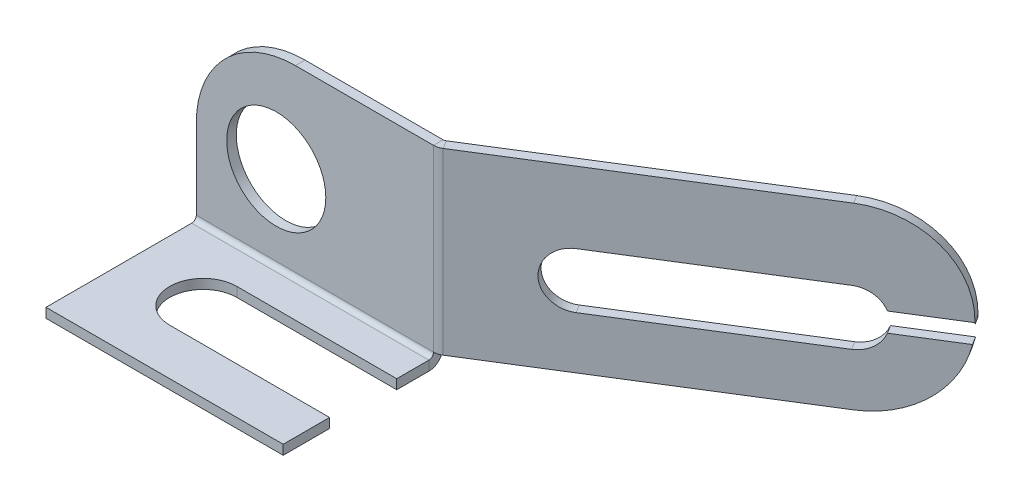
ISO-10303-21;
HEADER;
FILE_DESCRIPTION(('STEP AP214'),'2;1');
FILE_NAME('part.step','',(''),(''),'','','');
FILE_SCHEMA(('AUTOMOTIVE_DESIGN { 1 0 10303 214 1 1 1 1 }'));
ENDSEC;
DATA;
#1=APPLICATION_CONTEXT('core data for automotive mechanical design processes');
#2=APPLICATION_PROTOCOL_DEFINITION('international standard','automotive_design',2000,#1);
#3=PRODUCT_CONTEXT('',#1,'mechanical');
#4=PRODUCT('Part','Part','',(#3));
#5=PRODUCT_RELATED_PRODUCT_CATEGORY('part','',(#4));
#6=PRODUCT_DEFINITION_FORMATION('','',#4);
#7=PRODUCT_DEFINITION_CONTEXT('part definition',#1,'design');
#8=PRODUCT_DEFINITION('design','',#6,#7);
#9=PRODUCT_DEFINITION_SHAPE('','',#8);
#10=(LENGTH_UNIT() NAMED_UNIT(*) SI_UNIT(.MILLI.,.METRE.));
#11=(NAMED_UNIT(*) PLANE_ANGLE_UNIT() SI_UNIT($,.RADIAN.));
#12=(NAMED_UNIT(*) SI_UNIT($,.STERADIAN.) SOLID_ANGLE_UNIT());
#13=UNCERTAINTY_MEASURE_WITH_UNIT(LENGTH_MEASURE(1.E-05),#10,'distance_accuracy_value','');
#14=(GEOMETRIC_REPRESENTATION_CONTEXT(3) GLOBAL_UNCERTAINTY_ASSIGNED_CONTEXT((#13)) GLOBAL_UNIT_ASSIGNED_CONTEXT((#10,
#11,#12)) REPRESENTATION_CONTEXT('',''));
#15=CARTESIAN_POINT('',(0.,0.,0.));
#16=DIRECTION('',(0.,0.,1.));
#17=DIRECTION('',(1.,0.,0.));
#18=AXIS2_PLACEMENT_3D('',#15,#16,#17);
#19=CARTESIAN_POINT('',(37.6815119332738,23.1394,0.761999999999995));
#20=DIRECTION('',(1.,0.,0.));
#21=DIRECTION('',(0.,0.,-1.));
#22=AXIS2_PLACEMENT_3D('',#19,#20,#21);
#23=PLANE('',#22);
#24=DIRECTION('',(0.,1.,0.));
#25=VECTOR('',#24,1.);
#26=CARTESIAN_POINT('',(37.6815119332738,22.1234,6.604));
#27=LINE('',#26,#25);
#28=CARTESIAN_POINT('',(37.6815119332738,23.1394,6.604));
#29=VERTEX_POINT('',#28);
#30=CARTESIAN_POINT('',(37.6815119332738,24.6634,6.604));
#31=VERTEX_POINT('',#30);
#32=EDGE_CURVE('E267',#29,#31,#27,.T.);
#33=ORIENTED_EDGE('',*,*,#32,.F.);
#34=DIRECTION('',(0.,0.,-1.));
#35=VECTOR('',#34,1.);
#36=CARTESIAN_POINT('',(37.6815119332738,23.1394,0.761999999999995));
#37=LINE('',#36,#35);
#38=CARTESIAN_POINT('',(37.6815119332738,23.1394,1.49859999999999));
#39=VERTEX_POINT('',#38);
#40=EDGE_CURVE('E877',#29,#39,#37,.T.);
#41=ORIENTED_EDGE('',*,*,#40,.T.);
#42=DIRECTION('',(0.,-1.,0.));
#43=VECTOR('',#42,1.);
#44=CARTESIAN_POINT('',(37.6815119332738,24.6634,1.4986));
#45=LINE('',#44,#43);
#46=CARTESIAN_POINT('',(37.6815119332738,24.6634,1.4986));
#47=VERTEX_POINT('',#46);
#48=EDGE_CURVE('E283',#47,#39,#45,.T.);
#49=ORIENTED_EDGE('',*,*,#48,.F.);
#50=DIRECTION('',(0.,0.,1.));
#51=VECTOR('',#50,1.);
#52=CARTESIAN_POINT('',(37.6815119332738,24.6634,0.));
#53=LINE('',#52,#51);
#54=EDGE_CURVE('E271',#31,#47,#53,.F.);
#55=ORIENTED_EDGE('',*,*,#54,.F.);
#56=EDGE_LOOP('',(#33,#41,#49,#55));
#57=FACE_BOUND('',#56,.T.);
#58=ADVANCED_FACE('F69',(#57),#23,.T.);
#59=CARTESIAN_POINT('',(0.,12.7000000000001,-0.762));
#60=DIRECTION('',(-1.,0.,0.));
#61=DIRECTION('',(0.,0.,1.));
#62=AXIS2_PLACEMENT_3D('',#59,#60,#61);
#63=PLANE('',#62);
#64=DIRECTION('',(0.,-1.,0.));
#65=VECTOR('',#64,1.);
#66=CARTESIAN_POINT('',(0.,12.7000000000001,-0.762));
#67=LINE('',#66,#65);
#68=CARTESIAN_POINT('',(0.,38.0999999999999,-0.762));
#69=VERTEX_POINT('',#68);
#70=CARTESIAN_POINT('',(0.,25.4,-0.762));
#71=VERTEX_POINT('',#70);
#72=EDGE_CURVE('E351',#69,#71,#67,.T.);
#73=ORIENTED_EDGE('',*,*,#72,.T.);
#74=DIRECTION('',(0.,0.,1.));
#75=VECTOR('',#74,1.);
#76=CARTESIAN_POINT('',(0.,25.4,-0.762));
#77=LINE('',#76,#75);
#78=CARTESIAN_POINT('',(0.,25.4,0.761999999999998));
#79=VERTEX_POINT('',#78);
#80=EDGE_CURVE('E315',#79,#71,#77,.F.);
#81=ORIENTED_EDGE('',*,*,#80,.F.);
#82=DIRECTION('',(0.,-1.,0.));
#83=VECTOR('',#82,1.);
#84=CARTESIAN_POINT('',(0.,12.7000000000001,0.762));
#85=LINE('',#84,#83);
#86=CARTESIAN_POINT('',(0.,38.0999999999999,0.762));
#87=VERTEX_POINT('',#86);
#88=EDGE_CURVE('E336',#87,#79,#85,.T.);
#89=ORIENTED_EDGE('',*,*,#88,.F.);
#90=DIRECTION('',(0.,0.,1.));
#91=VECTOR('',#90,1.);
#92=CARTESIAN_POINT('',(0.,38.0999999999999,-0.762));
#93=LINE('',#92,#91);
#94=EDGE_CURVE('E356',#69,#87,#93,.T.);
#95=ORIENTED_EDGE('',*,*,#94,.F.);
#96=EDGE_LOOP('',(#73,#81,#89,#95));
#97=FACE_BOUND('',#96,.T.);
#98=ADVANCED_FACE('F511',(#97),#63,.T.);
#99=CARTESIAN_POINT('',(15.748,38.1,-0.762));
#100=DIRECTION('',(0.,0.,1.));
#101=DIRECTION('',(1.,0.,0.));
#102=AXIS2_PLACEMENT_3D('',#99,#100,#101);
#103=PLANE('',#102);
#104=CARTESIAN_POINT('',(12.7,38.1,-0.762));
#105=DIRECTION('',(0.,0.,1.));
#106=DIRECTION('',(1.,0.,0.));
#107=AXIS2_PLACEMENT_3D('',#104,#105,#106);
#108=CIRCLE('',#107,7.874);
#109=CARTESIAN_POINT('',(20.574,38.1,-0.762));
#110=VERTEX_POINT('',#109);
#111=EDGE_CURVE('E346',#110,#110,#108,.T.);
#112=ORIENTED_EDGE('',*,*,#111,.T.);
#113=EDGE_LOOP('',(#112));
#114=FACE_BOUND('',#113,.T.);
#115=DIRECTION('',(-1.,0.,0.));
#116=VECTOR('',#115,1.);
#117=CARTESIAN_POINT('',(15.748,25.4,-0.762));
#118=LINE('',#117,#116);
#119=CARTESIAN_POINT('',(37.6815119332738,25.4,-0.762000000000002));
#120=VERTEX_POINT('',#119);
#121=EDGE_CURVE('E307',#120,#71,#118,.T.);
#122=ORIENTED_EDGE('',*,*,#121,.T.);
#123=ORIENTED_EDGE('',*,*,#72,.F.);
#124=CARTESIAN_POINT('',(15.748,38.1,-0.762));
#125=DIRECTION('',(0.,0.,1.));
#126=DIRECTION('',(1.,0.,0.));
#127=AXIS2_PLACEMENT_3D('',#124,#125,#126);
#128=CIRCLE('',#127,15.748);
#129=CARTESIAN_POINT('',(15.7480000000001,53.848,-0.762));
#130=VERTEX_POINT('',#129);
#131=EDGE_CURVE('E359',#130,#69,#128,.T.);
#132=ORIENTED_EDGE('',*,*,#131,.F.);
#133=DIRECTION('',(-1.,0.,0.));
#134=VECTOR('',#133,1.);
#135=CARTESIAN_POINT('',(15.7480000000001,53.848,-0.762));
#136=LINE('',#135,#134);
#137=CARTESIAN_POINT('',(37.6815119332738,53.848,-0.762));
#138=VERTEX_POINT('',#137);
#139=EDGE_CURVE('E337',#138,#130,#136,.T.);
#140=ORIENTED_EDGE('',*,*,#139,.F.);
#141=DIRECTION('',(0.,-1.,0.));
#142=VECTOR('',#141,1.);
#143=CARTESIAN_POINT('',(37.6815119332738,38.1,-0.762));
#144=LINE('',#143,#142);
#145=EDGE_CURVE('E347',#138,#120,#144,.T.);
#146=ORIENTED_EDGE('',*,*,#145,.T.);
#147=EDGE_LOOP('',(#122,#123,#132,#140,#146));
#148=FACE_BOUND('',#147,.T.);
#149=ADVANCED_FACE('F519',(#114,#148),#103,.F.);
#150=CARTESIAN_POINT('',(15.748,38.1,0.762));
#151=DIRECTION('',(0.,0.,1.));
#152=DIRECTION('',(1.,0.,0.));
#153=AXIS2_PLACEMENT_3D('',#150,#151,#152);
#154=PLANE('',#153);
#155=CARTESIAN_POINT('',(12.7,38.1,0.762));
#156=DIRECTION('',(0.,0.,1.));
#157=DIRECTION('',(1.,0.,0.));
#158=AXIS2_PLACEMENT_3D('',#155,#156,#157);
#159=CIRCLE('',#158,7.874);
#160=CARTESIAN_POINT('',(20.574,38.1,0.762));
#161=VERTEX_POINT('',#160);
#162=EDGE_CURVE('E354',#161,#161,#159,.T.);
#163=ORIENTED_EDGE('',*,*,#162,.F.);
#164=EDGE_LOOP('',(#163));
#165=FACE_BOUND('',#164,.T.);
#166=ORIENTED_EDGE('',*,*,#88,.T.);
#167=DIRECTION('',(1.,0.,0.));
#168=VECTOR('',#167,1.);
#169=CARTESIAN_POINT('',(19.05,25.4,0.762));
#170=LINE('',#169,#168);
#171=CARTESIAN_POINT('',(37.6815119332738,25.4,0.761999999999998));
#172=VERTEX_POINT('',#171);
#173=EDGE_CURVE('E296',#172,#79,#170,.F.);
#174=ORIENTED_EDGE('',*,*,#173,.F.);
#175=DIRECTION('',(0.,-1.,0.));
#176=VECTOR('',#175,1.);
#177=CARTESIAN_POINT('',(37.6815119332738,38.1,0.762));
#178=LINE('',#177,#176);
#179=CARTESIAN_POINT('',(37.6815119332738,53.848,0.762));
#180=VERTEX_POINT('',#179);
#181=EDGE_CURVE('E361',#180,#172,#178,.T.);
#182=ORIENTED_EDGE('',*,*,#181,.F.);
#183=DIRECTION('',(-1.,0.,0.));
#184=VECTOR('',#183,1.);
#185=CARTESIAN_POINT('',(15.7480000000001,53.848,0.762));
#186=LINE('',#185,#184);
#187=CARTESIAN_POINT('',(15.7480000000001,53.848,0.762));
#188=VERTEX_POINT('',#187);
#189=EDGE_CURVE('E343',#180,#188,#186,.T.);
#190=ORIENTED_EDGE('',*,*,#189,.T.);
#191=CARTESIAN_POINT('',(15.748,38.1,0.762));
#192=DIRECTION('',(0.,0.,1.));
#193=DIRECTION('',(1.,0.,0.));
#194=AXIS2_PLACEMENT_3D('',#191,#192,#193);
#195=CIRCLE('',#194,15.748);
#196=EDGE_CURVE('E341',#188,#87,#195,.T.);
#197=ORIENTED_EDGE('',*,*,#196,.T.);
#198=EDGE_LOOP('',(#166,#174,#182,#190,#197));
#199=FACE_BOUND('',#198,.T.);
#200=ADVANCED_FACE('F500',(#165,#199),#154,.T.);
#201=CARTESIAN_POINT('',(37.6815119332738,71.797180792828,-1.4986));
#202=DIRECTION('',(0.,-1.,0.));
#203=DIRECTION('',(0.,0.,-1.));
#204=AXIS2_PLACEMENT_3D('',#201,#202,#203);
#205=CYLINDRICAL_SURFACE('',#204,0.7366);
#206=CARTESIAN_POINT('',(37.6815119332738,25.4,-1.4986));
#207=DIRECTION('',(0.,-1.,0.));
#208=DIRECTION('',(0.,0.,1.));
#209=AXIS2_PLACEMENT_3D('',#206,#207,#208);
#210=CIRCLE('',#209,0.7366);
#211=CARTESIAN_POINT('',(38.071850463308,25.4,-0.873927772371178));
#212=VERTEX_POINT('',#211);
#213=EDGE_CURVE('E322',#212,#120,#210,.T.);
#214=ORIENTED_EDGE('',*,*,#213,.T.);
#215=ORIENTED_EDGE('',*,*,#145,.F.);
#216=CARTESIAN_POINT('',(37.6815119332738,53.848,-1.4986));
#217=DIRECTION('',(0.,1.,0.));
#218=DIRECTION('',(0.,0.,-1.));
#219=AXIS2_PLACEMENT_3D('',#216,#217,#218);
#220=CIRCLE('',#219,0.7366);
#221=CARTESIAN_POINT('',(38.071850463308,53.848,-0.873927772371177));
#222=VERTEX_POINT('',#221);
#223=EDGE_CURVE('E318',#138,#222,#220,.T.);
#224=ORIENTED_EDGE('',*,*,#223,.T.);
#225=DIRECTION('',(0.,-1.,0.));
#226=VECTOR('',#225,1.);
#227=CARTESIAN_POINT('',(38.071850463308,38.1,-0.873927772371177));
#228=LINE('',#227,#226);
#229=EDGE_CURVE('E459',#222,#212,#228,.T.);
#230=ORIENTED_EDGE('',*,*,#229,.T.);
#231=EDGE_LOOP('',(#214,#215,#224,#230));
#232=FACE_BOUND('',#231,.T.);
#233=ADVANCED_FACE('F529',(#232),#205,.F.);
#234=CARTESIAN_POINT('',(37.6815119332738,71.797180792828,-1.4986));
#235=DIRECTION('',(0.,-1.,0.));
#236=DIRECTION('',(0.,0.,-1.));
#237=AXIS2_PLACEMENT_3D('',#234,#235,#236);
#238=CYLINDRICAL_SURFACE('',#237,2.2606);
#239=ORIENTED_EDGE('',*,*,#181,.T.);
#240=CARTESIAN_POINT('',(37.6815119332738,25.4,-1.4986));
#241=DIRECTION('',(0.,-1.,0.));
#242=DIRECTION('',(0.,0.,-1.));
#243=AXIS2_PLACEMENT_3D('',#240,#241,#242);
#244=CIRCLE('',#243,2.2606);
#245=CARTESIAN_POINT('',(38.8794474219994,25.4,0.418497526171215));
#246=VERTEX_POINT('',#245);
#247=EDGE_CURVE('E323',#246,#172,#244,.T.);
#248=ORIENTED_EDGE('',*,*,#247,.F.);
#249=DIRECTION('',(0.,-1.,0.));
#250=VECTOR('',#249,1.);
#251=CARTESIAN_POINT('',(38.8794474219994,38.1,0.418497526171215));
#252=LINE('',#251,#250);
#253=CARTESIAN_POINT('',(38.8794474219994,53.848,0.418497526171215));
#254=VERTEX_POINT('',#253);
#255=EDGE_CURVE('E77',#254,#246,#252,.T.);
#256=ORIENTED_EDGE('',*,*,#255,.F.);
#257=CARTESIAN_POINT('',(37.6815119332738,53.848,-1.4986));
#258=DIRECTION('',(0.,-1.,0.));
#259=DIRECTION('',(0.,0.,-1.));
#260=AXIS2_PLACEMENT_3D('',#257,#258,#259);
#261=CIRCLE('',#260,2.2606);
#262=EDGE_CURVE('E316',#180,#254,#261,.F.);
#263=ORIENTED_EDGE('',*,*,#262,.F.);
#264=EDGE_LOOP('',(#239,#248,#256,#263));
#265=FACE_BOUND('',#264,.T.);
#266=ADVANCED_FACE('F494',(#265),#238,.T.);
#267=CARTESIAN_POINT('',(78.2129451427182,25.4,-25.9568675896253));
#268=DIRECTION('',(0.,-1.,0.));
#269=DIRECTION('',(-0.529919264233206,0.,-0.848048096156425));
#270=AXIS2_PLACEMENT_3D('',#267,#268,#269);
#271=PLANE('',#270);
#272=DIRECTION('',(0.848048096156425,0.,-0.529919264233206));
#273=VECTOR('',#272,1.);
#274=CARTESIAN_POINT('',(79.0205421014096,25.4,-24.6644422910829));
#275=LINE('',#274,#273);
#276=CARTESIAN_POINT('',(79.0205421014096,25.4,-24.6644422910829));
#277=VERTEX_POINT('',#276);
#278=EDGE_CURVE('E428',#246,#277,#275,.T.);
#279=ORIENTED_EDGE('',*,*,#278,.F.);
#280=DIRECTION('',(-0.529919264233206,0.,-0.848048096156425));
#281=VECTOR('',#280,1.);
#282=CARTESIAN_POINT('',(38.071850463308,25.4,-0.873927772371177));
#283=LINE('',#282,#281);
#284=EDGE_CURVE('E458',#246,#212,#283,.T.);
#285=ORIENTED_EDGE('',*,*,#284,.T.);
#286=DIRECTION('',(0.848048096156425,0.,-0.529919264233206));
#287=VECTOR('',#286,1.);
#288=CARTESIAN_POINT('',(78.2129451427182,25.4,-25.9568675896253));
#289=LINE('',#288,#287);
#290=CARTESIAN_POINT('',(78.2129451427182,25.4,-25.9568675896253));
#291=VERTEX_POINT('',#290);
#292=EDGE_CURVE('E72',#212,#291,#289,.T.);
#293=ORIENTED_EDGE('',*,*,#292,.T.);
#294=DIRECTION('',(0.529919264233206,0.,0.848048096156425));
#295=VECTOR('',#294,1.);
#296=CARTESIAN_POINT('',(78.2129451427182,25.4,-25.9568675896253));
#297=LINE('',#296,#295);
#298=EDGE_CURVE('E455',#291,#277,#297,.T.);
#299=ORIENTED_EDGE('',*,*,#298,.T.);
#300=EDGE_LOOP('',(#279,#285,#293,#299));
#301=FACE_BOUND('',#300,.T.);
#302=ADVANCED_FACE('F466',(#301),#271,.T.);
#303=CARTESIAN_POINT('',(19.5689783684596,38.1,12.4850178087218));
#304=DIRECTION('',(0.529919264233206,0.,0.848048096156425));
#305=DIRECTION('',(0.848048096156425,0.,-0.529919264233206));
#306=AXIS2_PLACEMENT_3D('',#303,#304,#305);
#307=PLANE('',#306);
#308=DIRECTION('',(-0.848048096156425,0.,0.529919264233206));
#309=VECTOR('',#308,1.);
#310=CARTESIAN_POINT('',(19.5689783684597,53.848,12.4850178087217));
#311=LINE('',#310,#309);
#312=CARTESIAN_POINT('',(79.0205421014096,53.848,-24.6644422910829));
#313=VERTEX_POINT('',#312);
#314=EDGE_CURVE('E94',#313,#254,#311,.T.);
#315=ORIENTED_EDGE('',*,*,#314,.T.);
#316=ORIENTED_EDGE('',*,*,#255,.T.);
#317=ORIENTED_EDGE('',*,*,#278,.T.);
#318=CARTESIAN_POINT('',(79.0205421014097,39.37,-24.6644422910829));
#319=DIRECTION('',(0.529919264233206,0.,0.848048096156425));
#320=DIRECTION('',(0.848048096156425,0.,-0.529919264233206));
#321=AXIS2_PLACEMENT_3D('',#318,#319,#320);
#322=CIRCLE('',#321,13.97);
#323=CARTESIAN_POINT('',(90.6284113124176,36.576,-31.9178440020137));
#324=VERTEX_POINT('',#323);
#325=EDGE_CURVE('E440',#277,#324,#322,.T.);
#326=ORIENTED_EDGE('',*,*,#325,.T.);
#327=DIRECTION('',(0.848048096156425,0.,-0.529919264233206));
#328=VECTOR('',#327,1.);
#329=CARTESIAN_POINT('',(82.3080740718898,36.576,-26.718720262858));
#330=LINE('',#329,#328);
#331=CARTESIAN_POINT('',(82.3080740718898,36.576,-26.718720262858));
#332=VERTEX_POINT('',#331);
#333=EDGE_CURVE('E374',#332,#324,#330,.T.);
#334=ORIENTED_EDGE('',*,*,#333,.F.);
#335=CARTESIAN_POINT('',(78.805137884986,38.1,-24.5298427979677));
#336=DIRECTION('',(0.529919264233206,0.,0.848048096156425));
#337=DIRECTION('',(0.848048096156425,0.,-0.529919264233206));
#338=AXIS2_PLACEMENT_3D('',#335,#336,#337);
#339=CIRCLE('',#338,4.40276305129233);
#340=CARTESIAN_POINT('',(78.805137884986,33.6972369487077,-24.5298427979677));
#341=VERTEX_POINT('',#340);
#342=EDGE_CURVE('E375',#341,#332,#339,.T.);
#343=ORIENTED_EDGE('',*,*,#342,.F.);
#344=DIRECTION('',(0.848048096156425,0.,-0.529919264233206));
#345=VECTOR('',#344,1.);
#346=CARTESIAN_POINT('',(51.8796108320195,33.6972369487077,-7.70490615856339));
#347=LINE('',#346,#345);
#348=CARTESIAN_POINT('',(51.8796108320195,33.6972369487077,-7.7049061585634));
#349=VERTEX_POINT('',#348);
#350=EDGE_CURVE('E367',#349,#341,#347,.T.);
#351=ORIENTED_EDGE('',*,*,#350,.F.);
#352=CARTESIAN_POINT('',(51.8796108320195,38.1,-7.70490615856339));
#353=DIRECTION('',(0.529919264233206,0.,0.848048096156425));
#354=DIRECTION('',(0.848048096156425,0.,-0.529919264233206));
#355=AXIS2_PLACEMENT_3D('',#352,#353,#354);
#356=CIRCLE('',#355,4.40276305129234);
#357=CARTESIAN_POINT('',(51.8796108320195,42.5027630512923,-7.70490615856339));
#358=VERTEX_POINT('',#357);
#359=EDGE_CURVE('E331',#358,#349,#356,.T.);
#360=ORIENTED_EDGE('',*,*,#359,.F.);
#361=DIRECTION('',(0.848048096156425,0.,-0.529919264233206));
#362=VECTOR('',#361,1.);
#363=CARTESIAN_POINT('',(51.8796108320195,42.5027630512923,-7.70490615856339));
#364=LINE('',#363,#362);
#365=CARTESIAN_POINT('',(78.805137884986,42.5027630512923,-24.5298427979677));
#366=VERTEX_POINT('',#365);
#367=EDGE_CURVE('E384',#358,#366,#364,.T.);
#368=ORIENTED_EDGE('',*,*,#367,.T.);
#369=CARTESIAN_POINT('',(78.805137884986,38.1,-24.5298427979677));
#370=DIRECTION('',(0.529919264233206,0.,0.848048096156425));
#371=DIRECTION('',(0.848048096156425,0.,-0.529919264233206));
#372=AXIS2_PLACEMENT_3D('',#369,#370,#371);
#373=CIRCLE('',#372,4.40276305129233);
#374=CARTESIAN_POINT('',(82.3080740718898,39.624,-26.718720262858));
#375=VERTEX_POINT('',#374);
#376=EDGE_CURVE('E379',#375,#366,#373,.T.);
#377=ORIENTED_EDGE('',*,*,#376,.F.);
#378=DIRECTION('',(0.848048096156425,0.,-0.529919264233206));
#379=VECTOR('',#378,1.);
#380=CARTESIAN_POINT('',(82.3080740718898,39.624,-26.718720262858));
#381=LINE('',#380,#379);
#382=CARTESIAN_POINT('',(90.8658156227025,39.624,-32.0661906795219));
#383=VERTEX_POINT('',#382);
#384=EDGE_CURVE('E380',#375,#383,#381,.T.);
#385=ORIENTED_EDGE('',*,*,#384,.T.);
#386=CARTESIAN_POINT('',(79.0205421014097,39.37,-24.6644422910829));
#387=DIRECTION('',(0.529919264233206,0.,0.848048096156425));
#388=DIRECTION('',(0.848048096156425,0.,-0.529919264233206));
#389=AXIS2_PLACEMENT_3D('',#386,#387,#388);
#390=CIRCLE('',#389,13.97);
#391=CARTESIAN_POINT('',(90.8677740047149,39.37,-32.0674144124208));
#392=VERTEX_POINT('',#391);
#393=EDGE_CURVE('E450',#392,#383,#390,.T.);
#394=ORIENTED_EDGE('',*,*,#393,.F.);
#395=DIRECTION('',(0.,1.,0.));
#396=VECTOR('',#395,1.);
#397=CARTESIAN_POINT('',(90.8677740047149,39.8779999999999,-32.0674144124208));
#398=LINE('',#397,#396);
#399=CARTESIAN_POINT('',(90.8677740047149,39.8779999999999,-32.0674144124208));
#400=VERTEX_POINT('',#399);
#401=EDGE_CURVE('E439',#392,#400,#398,.T.);
#402=ORIENTED_EDGE('',*,*,#401,.T.);
#403=CARTESIAN_POINT('',(79.0205421014097,39.878,-24.6644422910829));
#404=DIRECTION('',(0.529919264233206,0.,0.848048096156425));
#405=DIRECTION('',(0.848048096156425,0.,-0.529919264233206));
#406=AXIS2_PLACEMENT_3D('',#403,#404,#405);
#407=CIRCLE('',#406,13.97);
#408=EDGE_CURVE('E442',#400,#313,#407,.T.);
#409=ORIENTED_EDGE('',*,*,#408,.T.);
#410=EDGE_LOOP('',(#315,#316,#317,#326,#334,#343,#351,#360,#368,#377,#385,#394,#402,#409));
#411=FACE_BOUND('',#410,.T.);
#412=ADVANCED_FACE('F481',(#411),#307,.T.);
#413=CARTESIAN_POINT('',(18.7613814097683,53.848,11.1925925101793));
#414=DIRECTION('',(0.,1.,0.));
#415=DIRECTION('',(0.529919264233206,0.,0.848048096156425));
#416=AXIS2_PLACEMENT_3D('',#413,#414,#415);
#417=PLANE('',#416);
#418=DIRECTION('',(-0.848048096156425,0.,0.529919264233206));
#419=VECTOR('',#418,1.);
#420=CARTESIAN_POINT('',(18.7613814097683,53.848,11.1925925101793));
#421=LINE('',#420,#419);
#422=CARTESIAN_POINT('',(78.2129451427182,53.848,-25.9568675896253));
#423=VERTEX_POINT('',#422);
#424=EDGE_CURVE('E436',#423,#222,#421,.T.);
#425=ORIENTED_EDGE('',*,*,#424,.T.);
#426=DIRECTION('',(0.529919264233206,0.,0.848048096156425));
#427=VECTOR('',#426,1.);
#428=CARTESIAN_POINT('',(38.071850463308,53.848,-0.873927772371177));
#429=LINE('',#428,#427);
#430=EDGE_CURVE('E13',#222,#254,#429,.T.);
#431=ORIENTED_EDGE('',*,*,#430,.T.);
#432=ORIENTED_EDGE('',*,*,#314,.F.);
#433=DIRECTION('',(0.529919264233206,0.,0.848048096156425));
#434=VECTOR('',#433,1.);
#435=CARTESIAN_POINT('',(78.2129451427182,53.848,-25.9568675896253));
#436=LINE('',#435,#434);
#437=EDGE_CURVE('E444',#423,#313,#436,.T.);
#438=ORIENTED_EDGE('',*,*,#437,.F.);
#439=EDGE_LOOP('',(#425,#431,#432,#438));
#440=FACE_BOUND('',#439,.T.);
#441=ADVANCED_FACE('F66',(#440),#417,.T.);
#442=CARTESIAN_POINT('',(18.7613814097682,38.1,11.1925925101794));
#443=DIRECTION('',(0.529919264233206,0.,0.848048096156425));
#444=DIRECTION('',(0.848048096156425,0.,-0.529919264233206));
#445=AXIS2_PLACEMENT_3D('',#442,#443,#444);
#446=PLANE('',#445);
#447=ORIENTED_EDGE('',*,*,#229,.F.);
#448=ORIENTED_EDGE('',*,*,#424,.F.);
#449=CARTESIAN_POINT('',(78.2129451427183,39.878,-25.9568675896253));
#450=DIRECTION('',(0.529919264233206,0.,0.848048096156425));
#451=DIRECTION('',(0.848048096156425,0.,-0.529919264233206));
#452=AXIS2_PLACEMENT_3D('',#449,#450,#451);
#453=CIRCLE('',#452,13.97);
#454=CARTESIAN_POINT('',(90.0601770460236,39.8779999999999,-33.3598397109632));
#455=VERTEX_POINT('',#454);
#456=EDGE_CURVE('E433',#455,#423,#453,.T.);
#457=ORIENTED_EDGE('',*,*,#456,.F.);
#458=DIRECTION('',(0.,1.,0.));
#459=VECTOR('',#458,1.);
#460=CARTESIAN_POINT('',(90.0601770460236,39.8779999999999,-33.3598397109632));
#461=LINE('',#460,#459);
#462=CARTESIAN_POINT('',(90.0601770460236,39.37,-33.3598397109632));
#463=VERTEX_POINT('',#462);
#464=EDGE_CURVE('E427',#463,#455,#461,.T.);
#465=ORIENTED_EDGE('',*,*,#464,.F.);
#466=CARTESIAN_POINT('',(78.2129451427183,39.37,-25.9568675896253));
#467=DIRECTION('',(0.529919264233206,0.,0.848048096156425));
#468=DIRECTION('',(0.848048096156425,0.,-0.529919264233206));
#469=AXIS2_PLACEMENT_3D('',#466,#467,#468);
#470=CIRCLE('',#469,13.97);
#471=CARTESIAN_POINT('',(90.0582186640111,39.624,-33.3586159780643));
#472=VERTEX_POINT('',#471);
#473=EDGE_CURVE('E415',#463,#472,#470,.T.);
#474=ORIENTED_EDGE('',*,*,#473,.T.);
#475=DIRECTION('',(0.848048096156425,0.,-0.529919264233206));
#476=VECTOR('',#475,1.);
#477=CARTESIAN_POINT('',(18.7613814097682,39.624,11.1925925101794));
#478=LINE('',#477,#476);
#479=CARTESIAN_POINT('',(81.5004771131984,39.624,-28.0111455614004));
#480=VERTEX_POINT('',#479);
#481=EDGE_CURVE('E418',#480,#472,#478,.T.);
#482=ORIENTED_EDGE('',*,*,#481,.F.);
#483=CARTESIAN_POINT('',(77.9975409262946,38.1,-25.8222680965101));
#484=DIRECTION('',(0.529919264233206,0.,0.848048096156425));
#485=DIRECTION('',(0.848048096156425,0.,-0.529919264233206));
#486=AXIS2_PLACEMENT_3D('',#483,#484,#485);
#487=CIRCLE('',#486,4.40276305129233);
#488=CARTESIAN_POINT('',(77.9975409262946,42.5027630512923,-25.8222680965101));
#489=VERTEX_POINT('',#488);
#490=EDGE_CURVE('E417',#480,#489,#487,.T.);
#491=ORIENTED_EDGE('',*,*,#490,.T.);
#492=DIRECTION('',(0.848048096156425,0.,-0.529919264233206));
#493=VECTOR('',#492,1.);
#494=CARTESIAN_POINT('',(18.7613814097682,42.5027630512923,11.1925925101794));
#495=LINE('',#494,#493);
#496=CARTESIAN_POINT('',(51.072013873328,42.5027630512923,-8.99733145710579));
#497=VERTEX_POINT('',#496);
#498=EDGE_CURVE('E423',#497,#489,#495,.T.);
#499=ORIENTED_EDGE('',*,*,#498,.F.);
#500=CARTESIAN_POINT('',(51.072013873328,38.1,-8.99733145710579));
#501=DIRECTION('',(0.529919264233206,0.,0.848048096156425));
#502=DIRECTION('',(0.848048096156425,0.,-0.529919264233206));
#503=AXIS2_PLACEMENT_3D('',#500,#501,#502);
#504=CIRCLE('',#503,4.40276305129234);
#505=CARTESIAN_POINT('',(51.072013873328,33.6972369487077,-8.99733145710579));
#506=VERTEX_POINT('',#505);
#507=EDGE_CURVE('E421',#497,#506,#504,.T.);
#508=ORIENTED_EDGE('',*,*,#507,.T.);
#509=DIRECTION('',(0.848048096156425,0.,-0.529919264233206));
#510=VECTOR('',#509,1.);
#511=CARTESIAN_POINT('',(18.7613814097682,33.6972369487077,11.1925925101794));
#512=LINE('',#511,#510);
#513=CARTESIAN_POINT('',(77.9975409262946,33.6972369487077,-25.8222680965101));
#514=VERTEX_POINT('',#513);
#515=EDGE_CURVE('E388',#506,#514,#512,.T.);
#516=ORIENTED_EDGE('',*,*,#515,.T.);
#517=CARTESIAN_POINT('',(77.9975409262946,38.1,-25.8222680965101));
#518=DIRECTION('',(0.529919264233206,0.,0.848048096156425));
#519=DIRECTION('',(0.848048096156425,0.,-0.529919264233206));
#520=AXIS2_PLACEMENT_3D('',#517,#518,#519);
#521=CIRCLE('',#520,4.40276305129233);
#522=CARTESIAN_POINT('',(81.5004771131984,36.576,-28.0111455614004));
#523=VERTEX_POINT('',#522);
#524=EDGE_CURVE('E410',#514,#523,#521,.T.);
#525=ORIENTED_EDGE('',*,*,#524,.T.);
#526=DIRECTION('',(0.848048096156425,0.,-0.529919264233206));
#527=VECTOR('',#526,1.);
#528=CARTESIAN_POINT('',(18.7613814097682,36.576,11.1925925101794));
#529=LINE('',#528,#527);
#530=CARTESIAN_POINT('',(89.8208143537262,36.576,-33.2102693005561));
#531=VERTEX_POINT('',#530);
#532=EDGE_CURVE('E409',#523,#531,#529,.T.);
#533=ORIENTED_EDGE('',*,*,#532,.T.);
#534=CARTESIAN_POINT('',(78.2129451427183,39.37,-25.9568675896253));
#535=DIRECTION('',(0.529919264233206,0.,0.848048096156425));
#536=DIRECTION('',(0.848048096156425,0.,-0.529919264233206));
#537=AXIS2_PLACEMENT_3D('',#534,#535,#536);
#538=CIRCLE('',#537,13.97);
#539=EDGE_CURVE('E430',#291,#531,#538,.T.);
#540=ORIENTED_EDGE('',*,*,#539,.F.);
#541=ORIENTED_EDGE('',*,*,#292,.F.);
#542=EDGE_LOOP('',(#447,#448,#457,#465,#474,#482,#491,#499,#508,#516,#525,#533,#540,#541));
#543=FACE_BOUND('',#542,.T.);
#544=ADVANCED_FACE('F474',(#543),#446,.F.);
#545=CARTESIAN_POINT('',(78.2129451427183,39.878,-25.9568675896253));
#546=DIRECTION('',(0.529919264233206,0.,0.848048096156425));
#547=DIRECTION('',(0.848048096156425,0.,-0.529919264233206));
#548=AXIS2_PLACEMENT_3D('',#545,#546,#547);
#549=CYLINDRICAL_SURFACE('',#548,13.97);
#550=ORIENTED_EDGE('',*,*,#408,.F.);
#551=DIRECTION('',(0.529919264233206,0.,0.848048096156425));
#552=VECTOR('',#551,1.);
#553=CARTESIAN_POINT('',(90.0601770460236,39.8779999999999,-33.3598397109632));
#554=LINE('',#553,#552);
#555=EDGE_CURVE('E449',#455,#400,#554,.T.);
#556=ORIENTED_EDGE('',*,*,#555,.F.);
#557=ORIENTED_EDGE('',*,*,#456,.T.);
#558=ORIENTED_EDGE('',*,*,#437,.T.);
#559=EDGE_LOOP('',(#550,#556,#557,#558));
#560=FACE_BOUND('',#559,.T.);
#561=ADVANCED_FACE('F533',(#560),#549,.T.);
#562=CARTESIAN_POINT('',(90.0601770460236,39.8779999999999,-33.3598397109632));
#563=DIRECTION('',(0.848048096156425,0.,-0.529919264233206));
#564=DIRECTION('',(-0.529919264233206,0.,-0.848048096156425));
#565=AXIS2_PLACEMENT_3D('',#562,#563,#564);
#566=PLANE('',#565);
#567=ORIENTED_EDGE('',*,*,#401,.F.);
#568=DIRECTION('',(0.529919264233206,0.,0.848048096156425));
#569=VECTOR('',#568,1.);
#570=CARTESIAN_POINT('',(90.0601770460236,39.3700000000001,-33.3598397109632));
#571=LINE('',#570,#569);
#572=EDGE_CURVE('E448',#463,#392,#571,.T.);
#573=ORIENTED_EDGE('',*,*,#572,.F.);
#574=ORIENTED_EDGE('',*,*,#464,.T.);
#575=ORIENTED_EDGE('',*,*,#555,.T.);
#576=EDGE_LOOP('',(#567,#573,#574,#575));
#577=FACE_BOUND('',#576,.T.);
#578=ADVANCED_FACE('F539',(#577),#566,.T.);
#579=CARTESIAN_POINT('',(78.2129451427183,39.37,-25.9568675896253));
#580=DIRECTION('',(0.529919264233206,0.,0.848048096156425));
#581=DIRECTION('',(0.848048096156425,0.,-0.529919264233206));
#582=AXIS2_PLACEMENT_3D('',#579,#580,#581);
#583=CYLINDRICAL_SURFACE('',#582,13.97);
#584=DIRECTION('',(0.529919264233206,0.,0.848048096156425));
#585=VECTOR('',#584,1.);
#586=CARTESIAN_POINT('',(89.2824163812653,36.576,-34.071886166251));
#587=LINE('',#586,#585);
#588=EDGE_CURVE('E397',#531,#324,#587,.T.);
#589=ORIENTED_EDGE('',*,*,#588,.T.);
#590=ORIENTED_EDGE('',*,*,#325,.F.);
#591=ORIENTED_EDGE('',*,*,#298,.F.);
#592=ORIENTED_EDGE('',*,*,#539,.T.);
#593=EDGE_LOOP('',(#589,#590,#591,#592));
#594=FACE_BOUND('',#593,.T.);
#595=ADVANCED_FACE('F473',(#594),#583,.T.);
#596=CARTESIAN_POINT('',(50.5336159008671,38.1,-9.85894832280071));
#597=DIRECTION('',(0.529919264233206,0.,0.848048096156425));
#598=DIRECTION('',(0.848048096156425,0.,-0.529919264233206));
#599=AXIS2_PLACEMENT_3D('',#596,#597,#598);
#600=CYLINDRICAL_SURFACE('',#599,4.40276305129234);
#601=DIRECTION('',(0.529919264233206,0.,0.848048096156425));
#602=VECTOR('',#601,1.);
#603=CARTESIAN_POINT('',(50.5336159008671,42.5027630512923,-9.85894832280071));
#604=LINE('',#603,#602);
#605=EDGE_CURVE('E390',#497,#358,#604,.T.);
#606=ORIENTED_EDGE('',*,*,#605,.T.);
#607=ORIENTED_EDGE('',*,*,#359,.T.);
#608=DIRECTION('',(0.529919264233206,0.,0.848048096156425));
#609=VECTOR('',#608,1.);
#610=CARTESIAN_POINT('',(50.5336159008671,33.6972369487077,-9.85894832280071));
#611=LINE('',#610,#609);
#612=EDGE_CURVE('E386',#506,#349,#611,.T.);
#613=ORIENTED_EDGE('',*,*,#612,.F.);
#614=ORIENTED_EDGE('',*,*,#507,.F.);
#615=EDGE_LOOP('',(#606,#607,#613,#614));
#616=FACE_BOUND('',#615,.T.);
#617=ADVANCED_FACE('F561',(#616),#600,.F.);
#618=CARTESIAN_POINT('',(50.5336159008671,42.5027630512923,-9.85894832280071));
#619=DIRECTION('',(0.,-1.,0.));
#620=DIRECTION('',(-0.529919264233206,0.,-0.848048096156425));
#621=AXIS2_PLACEMENT_3D('',#618,#619,#620);
#622=PLANE('',#621);
#623=ORIENTED_EDGE('',*,*,#498,.T.);
#624=DIRECTION('',(0.529919264233206,0.,0.848048096156425));
#625=VECTOR('',#624,1.);
#626=CARTESIAN_POINT('',(77.4591429538336,42.5027630512923,-26.683884962205));
#627=LINE('',#626,#625);
#628=EDGE_CURVE('E389',#489,#366,#627,.T.);
#629=ORIENTED_EDGE('',*,*,#628,.T.);
#630=ORIENTED_EDGE('',*,*,#367,.F.);
#631=ORIENTED_EDGE('',*,*,#605,.F.);
#632=EDGE_LOOP('',(#623,#629,#630,#631));
#633=FACE_BOUND('',#632,.T.);
#634=ADVANCED_FACE('F560',(#633),#622,.T.);
#635=CARTESIAN_POINT('',(77.4591429538336,38.1,-26.683884962205));
#636=DIRECTION('',(0.529919264233206,0.,0.848048096156425));
#637=DIRECTION('',(0.848048096156425,0.,-0.529919264233206));
#638=AXIS2_PLACEMENT_3D('',#635,#636,#637);
#639=CYLINDRICAL_SURFACE('',#638,4.40276305129233);
#640=DIRECTION('',(0.529919264233206,0.,0.848048096156425));
#641=VECTOR('',#640,1.);
#642=CARTESIAN_POINT('',(80.9620791407374,39.624,-28.8727624270953));
#643=LINE('',#642,#641);
#644=EDGE_CURVE('E394',#480,#375,#643,.T.);
#645=ORIENTED_EDGE('',*,*,#644,.T.);
#646=ORIENTED_EDGE('',*,*,#376,.T.);
#647=ORIENTED_EDGE('',*,*,#628,.F.);
#648=ORIENTED_EDGE('',*,*,#490,.F.);
#649=EDGE_LOOP('',(#645,#646,#647,#648));
#650=FACE_BOUND('',#649,.T.);
#651=ADVANCED_FACE('F555',(#650),#639,.F.);
#652=CARTESIAN_POINT('',(80.9620791407374,39.624,-28.8727624270953));
#653=DIRECTION('',(0.,-1.,0.));
#654=DIRECTION('',(-0.529919264233206,0.,-0.848048096156425));
#655=AXIS2_PLACEMENT_3D('',#652,#653,#654);
#656=PLANE('',#655);
#657=ORIENTED_EDGE('',*,*,#481,.T.);
#658=DIRECTION('',(0.529919264233206,0.,0.848048096156425));
#659=VECTOR('',#658,1.);
#660=CARTESIAN_POINT('',(89.5198206915502,39.624,-34.2202328437592));
#661=LINE('',#660,#659);
#662=EDGE_CURVE('E391',#472,#383,#661,.T.);
#663=ORIENTED_EDGE('',*,*,#662,.T.);
#664=ORIENTED_EDGE('',*,*,#384,.F.);
#665=ORIENTED_EDGE('',*,*,#644,.F.);
#666=EDGE_LOOP('',(#657,#663,#664,#665));
#667=FACE_BOUND('',#666,.T.);
#668=ADVANCED_FACE('F550',(#667),#656,.T.);
#669=CARTESIAN_POINT('',(77.6745471702574,39.37,-26.8184844553202));
#670=DIRECTION('',(0.529919264233206,0.,0.848048096156425));
#671=DIRECTION('',(0.848048096156425,0.,-0.529919264233206));
#672=AXIS2_PLACEMENT_3D('',#669,#670,#671);
#673=CYLINDRICAL_SURFACE('',#672,13.97);
#674=ORIENTED_EDGE('',*,*,#572,.T.);
#675=ORIENTED_EDGE('',*,*,#393,.T.);
#676=ORIENTED_EDGE('',*,*,#662,.F.);
#677=ORIENTED_EDGE('',*,*,#473,.F.);
#678=EDGE_LOOP('',(#674,#675,#676,#677));
#679=FACE_BOUND('',#678,.T.);
#680=ADVANCED_FACE('F545',(#679),#673,.F.);
#681=CARTESIAN_POINT('',(80.9620791407374,36.576,-28.8727624270953));
#682=DIRECTION('',(0.,-1.,0.));
#683=DIRECTION('',(-0.529919264233206,0.,-0.848048096156425));
#684=AXIS2_PLACEMENT_3D('',#681,#682,#683);
#685=PLANE('',#684);
#686=DIRECTION('',(0.529919264233206,0.,0.848048096156425));
#687=VECTOR('',#686,1.);
#688=CARTESIAN_POINT('',(80.9620791407374,36.576,-28.8727624270953));
#689=LINE('',#688,#687);
#690=EDGE_CURVE('E399',#523,#332,#689,.T.);
#691=ORIENTED_EDGE('',*,*,#690,.T.);
#692=ORIENTED_EDGE('',*,*,#333,.T.);
#693=ORIENTED_EDGE('',*,*,#588,.F.);
#694=ORIENTED_EDGE('',*,*,#532,.F.);
#695=EDGE_LOOP('',(#691,#692,#693,#694));
#696=FACE_BOUND('',#695,.T.);
#697=ADVANCED_FACE('F480',(#696),#685,.F.);
#698=CARTESIAN_POINT('',(77.4591429538336,38.1,-26.683884962205));
#699=DIRECTION('',(0.529919264233206,0.,0.848048096156425));
#700=DIRECTION('',(0.848048096156425,0.,-0.529919264233206));
#701=AXIS2_PLACEMENT_3D('',#698,#699,#700);
#702=CYLINDRICAL_SURFACE('',#701,4.40276305129233);
#703=DIRECTION('',(0.529919264233206,0.,0.848048096156425));
#704=VECTOR('',#703,1.);
#705=CARTESIAN_POINT('',(77.4591429538336,33.6972369487077,-26.683884962205));
#706=LINE('',#705,#704);
#707=EDGE_CURVE('E402',#514,#341,#706,.T.);
#708=ORIENTED_EDGE('',*,*,#707,.T.);
#709=ORIENTED_EDGE('',*,*,#342,.T.);
#710=ORIENTED_EDGE('',*,*,#690,.F.);
#711=ORIENTED_EDGE('',*,*,#524,.F.);
#712=EDGE_LOOP('',(#708,#709,#710,#711));
#713=FACE_BOUND('',#712,.T.);
#714=ADVANCED_FACE('F478',(#713),#702,.F.);
#715=CARTESIAN_POINT('',(50.5336159008671,33.6972369487077,-9.85894832280071));
#716=DIRECTION('',(0.,-1.,0.));
#717=DIRECTION('',(-0.529919264233206,0.,-0.848048096156425));
#718=AXIS2_PLACEMENT_3D('',#715,#716,#717);
#719=PLANE('',#718);
#720=ORIENTED_EDGE('',*,*,#612,.T.);
#721=ORIENTED_EDGE('',*,*,#350,.T.);
#722=ORIENTED_EDGE('',*,*,#707,.F.);
#723=ORIENTED_EDGE('',*,*,#515,.F.);
#724=EDGE_LOOP('',(#720,#721,#722,#723));
#725=FACE_BOUND('',#724,.T.);
#726=ADVANCED_FACE('F562',(#725),#719,.F.);
#727=CARTESIAN_POINT('',(15.748,38.1,-0.762));
#728=DIRECTION('',(0.,0.,1.));
#729=DIRECTION('',(1.,0.,0.));
#730=AXIS2_PLACEMENT_3D('',#727,#728,#729);
#731=CYLINDRICAL_SURFACE('',#730,15.748);
#732=ORIENTED_EDGE('',*,*,#196,.F.);
#733=DIRECTION('',(0.,0.,1.));
#734=VECTOR('',#733,1.);
#735=CARTESIAN_POINT('',(15.7480000000001,53.848,-0.762));
#736=LINE('',#735,#734);
#737=EDGE_CURVE('E335',#130,#188,#736,.T.);
#738=ORIENTED_EDGE('',*,*,#737,.F.);
#739=ORIENTED_EDGE('',*,*,#131,.T.);
#740=ORIENTED_EDGE('',*,*,#94,.T.);
#741=EDGE_LOOP('',(#732,#738,#739,#740));
#742=FACE_BOUND('',#741,.T.);
#743=ADVANCED_FACE('F509',(#742),#731,.T.);
#744=CARTESIAN_POINT('',(12.7,38.1,-1.778));
#745=DIRECTION('',(0.,0.,1.));
#746=DIRECTION('',(1.,0.,0.));
#747=AXIS2_PLACEMENT_3D('',#744,#745,#746);
#748=CYLINDRICAL_SURFACE('',#747,7.874);
#749=ORIENTED_EDGE('',*,*,#162,.T.);
#750=EDGE_LOOP('',(#749));
#751=FACE_BOUND('',#750,.T.);
#752=ORIENTED_EDGE('',*,*,#111,.F.);
#753=EDGE_LOOP('',(#752));
#754=FACE_BOUND('',#753,.T.);
#755=ADVANCED_FACE('F571',(#751,#754),#748,.F.);
#756=CARTESIAN_POINT('',(15.7480000000001,53.848,-0.762));
#757=DIRECTION('',(0.,1.,0.));
#758=DIRECTION('',(0.,0.,1.));
#759=AXIS2_PLACEMENT_3D('',#756,#757,#758);
#760=PLANE('',#759);
#761=DIRECTION('',(0.,0.,1.));
#762=VECTOR('',#761,1.);
#763=CARTESIAN_POINT('',(37.6815119332738,53.848,-0.762));
#764=LINE('',#763,#762);
#765=EDGE_CURVE('E329',#138,#180,#764,.T.);
#766=ORIENTED_EDGE('',*,*,#765,.F.);
#767=ORIENTED_EDGE('',*,*,#139,.T.);
#768=ORIENTED_EDGE('',*,*,#737,.T.);
#769=ORIENTED_EDGE('',*,*,#189,.F.);
#770=EDGE_LOOP('',(#766,#767,#768,#769));
#771=FACE_BOUND('',#770,.T.);
#772=ADVANCED_FACE('F504',(#771),#760,.T.);
#773=CARTESIAN_POINT('',(37.6815119332738,53.848,-1.4986));
#774=DIRECTION('',(0.,-1.,0.));
#775=DIRECTION('',(0.,0.,-1.));
#776=AXIS2_PLACEMENT_3D('',#773,#774,#775);
#777=PLANE('',#776);
#778=ORIENTED_EDGE('',*,*,#765,.T.);
#779=ORIENTED_EDGE('',*,*,#262,.T.);
#780=ORIENTED_EDGE('',*,*,#430,.F.);
#781=ORIENTED_EDGE('',*,*,#223,.F.);
#782=EDGE_LOOP('',(#778,#779,#780,#781));
#783=FACE_BOUND('',#782,.T.);
#784=ADVANCED_FACE('F501',(#783),#777,.F.);
#785=CARTESIAN_POINT('',(37.6815119332738,25.4,-1.4986));
#786=DIRECTION('',(0.,1.,0.));
#787=DIRECTION('',(0.,0.,1.));
#788=AXIS2_PLACEMENT_3D('',#785,#786,#787);
#789=PLANE('',#788);
#790=ORIENTED_EDGE('',*,*,#284,.F.);
#791=ORIENTED_EDGE('',*,*,#247,.T.);
#792=DIRECTION('',(0.,0.,1.));
#793=VECTOR('',#792,1.);
#794=CARTESIAN_POINT('',(37.6815119332738,25.4,0.762));
#795=LINE('',#794,#793);
#796=EDGE_CURVE('E317',#172,#120,#795,.F.);
#797=ORIENTED_EDGE('',*,*,#796,.T.);
#798=ORIENTED_EDGE('',*,*,#213,.F.);
#799=EDGE_LOOP('',(#790,#791,#797,#798));
#800=FACE_BOUND('',#799,.T.);
#801=ADVANCED_FACE('F495',(#800),#789,.F.);
#802=CARTESIAN_POINT('',(0.,25.4,1.4986));
#803=DIRECTION('',(-1.,0.,0.));
#804=DIRECTION('',(0.,0.,1.));
#805=AXIS2_PLACEMENT_3D('',#802,#803,#804);
#806=PLANE('',#805);
#807=DIRECTION('',(0.,-1.,0.));
#808=VECTOR('',#807,1.);
#809=CARTESIAN_POINT('',(0.,23.1394,1.49859999999999));
#810=LINE('',#809,#808);
#811=CARTESIAN_POINT('',(0.,24.6634,1.4986));
#812=VERTEX_POINT('',#811);
#813=CARTESIAN_POINT('',(0.,23.1394,1.49859999999999));
#814=VERTEX_POINT('',#813);
#815=EDGE_CURVE('E293',#812,#814,#810,.T.);
#816=ORIENTED_EDGE('',*,*,#815,.F.);
#817=CARTESIAN_POINT('',(0.,25.4,1.4986));
#818=DIRECTION('',(1.,0.,0.));
#819=DIRECTION('',(0.,0.,-1.));
#820=AXIS2_PLACEMENT_3D('',#817,#818,#819);
#821=CIRCLE('',#820,0.7366);
#822=EDGE_CURVE('E305',#79,#812,#821,.F.);
#823=ORIENTED_EDGE('',*,*,#822,.F.);
#824=ORIENTED_EDGE('',*,*,#80,.T.);
#825=CARTESIAN_POINT('',(0.,25.4,1.4986));
#826=DIRECTION('',(1.,0.,0.));
#827=DIRECTION('',(0.,0.,-1.));
#828=AXIS2_PLACEMENT_3D('',#825,#826,#827);
#829=CIRCLE('',#828,2.2606);
#830=EDGE_CURVE('E294',#71,#814,#829,.F.);
#831=ORIENTED_EDGE('',*,*,#830,.T.);
#832=EDGE_LOOP('',(#816,#823,#824,#831));
#833=FACE_BOUND('',#832,.T.);
#834=ADVANCED_FACE('F517',(#833),#806,.T.);
#835=CARTESIAN_POINT('',(37.6815119332738,25.4,1.4986));
#836=DIRECTION('',(-1.,0.,0.));
#837=DIRECTION('',(0.,0.,1.));
#838=AXIS2_PLACEMENT_3D('',#835,#836,#837);
#839=PLANE('',#838);
#840=CARTESIAN_POINT('',(37.6815119332738,25.4,1.4986));
#841=DIRECTION('',(1.,0.,0.));
#842=DIRECTION('',(0.,0.,-1.));
#843=AXIS2_PLACEMENT_3D('',#840,#841,#842);
#844=CIRCLE('',#843,0.7366);
#845=EDGE_CURVE('E304',#47,#172,#844,.T.);
#846=ORIENTED_EDGE('',*,*,#845,.F.);
#847=ORIENTED_EDGE('',*,*,#48,.T.);
#848=CARTESIAN_POINT('',(37.6815119332738,25.4,1.4986));
#849=DIRECTION('',(1.,0.,0.));
#850=DIRECTION('',(0.,0.,-1.));
#851=AXIS2_PLACEMENT_3D('',#848,#849,#850);
#852=CIRCLE('',#851,2.2606);
#853=EDGE_CURVE('E299',#39,#120,#852,.T.);
#854=ORIENTED_EDGE('',*,*,#853,.T.);
#855=ORIENTED_EDGE('',*,*,#796,.F.);
#856=EDGE_LOOP('',(#846,#847,#854,#855));
#857=FACE_BOUND('',#856,.T.);
#858=ADVANCED_FACE('F527',(#857),#839,.F.);
#859=CARTESIAN_POINT('',(37.6815119332738,25.4,1.4986));
#860=DIRECTION('',(1.,0.,0.));
#861=DIRECTION('',(0.,-1.,0.));
#862=AXIS2_PLACEMENT_3D('',#859,#860,#861);
#863=CYLINDRICAL_SURFACE('',#862,2.2606);
#864=ORIENTED_EDGE('',*,*,#121,.F.);
#865=ORIENTED_EDGE('',*,*,#853,.F.);
#866=DIRECTION('',(1.,0.,0.));
#867=VECTOR('',#866,1.);
#868=CARTESIAN_POINT('',(0.,23.1394,1.49859999999999));
#869=LINE('',#868,#867);
#870=EDGE_CURVE('E284',#814,#39,#869,.T.);
#871=ORIENTED_EDGE('',*,*,#870,.F.);
#872=ORIENTED_EDGE('',*,*,#830,.F.);
#873=EDGE_LOOP('',(#864,#865,#871,#872));
#874=FACE_BOUND('',#873,.T.);
#875=ADVANCED_FACE('F525',(#874),#863,.T.);
#876=CARTESIAN_POINT('',(37.6815119332738,25.4,1.4986));
#877=DIRECTION('',(1.,0.,0.));
#878=DIRECTION('',(0.,-1.,0.));
#879=AXIS2_PLACEMENT_3D('',#876,#877,#878);
#880=CYLINDRICAL_SURFACE('',#879,0.7366);
#881=ORIENTED_EDGE('',*,*,#173,.T.);
#882=ORIENTED_EDGE('',*,*,#822,.T.);
#883=DIRECTION('',(-1.,0.,0.));
#884=VECTOR('',#883,1.);
#885=CARTESIAN_POINT('',(0.,24.6634,1.4986));
#886=LINE('',#885,#884);
#887=EDGE_CURVE('E287',#812,#47,#886,.F.);
#888=ORIENTED_EDGE('',*,*,#887,.T.);
#889=ORIENTED_EDGE('',*,*,#845,.T.);
#890=EDGE_LOOP('',(#881,#882,#888,#889));
#891=FACE_BOUND('',#890,.T.);
#892=ADVANCED_FACE('F590',(#891),#880,.F.);
#893=DIRECTION('',(0.,1.,0.));
#894=VECTOR('',#893,1.);
#895=CARTESIAN_POINT('',(37.6815119332738,22.1233999999999,17.272));
#896=LINE('',#895,#894);
#897=CARTESIAN_POINT('',(37.6815119332738,23.1393999999999,17.272));
#898=VERTEX_POINT('',#897);
#899=CARTESIAN_POINT('',(37.6815119332738,24.6633999999999,17.272));
#900=VERTEX_POINT('',#899);
#901=EDGE_CURVE('E255',#898,#900,#896,.T.);
#902=ORIENTED_EDGE('',*,*,#901,.T.);
#903=CARTESIAN_POINT('',(37.6815119332738,24.6633999999999,24.638));
#904=VERTEX_POINT('',#903);
#905=EDGE_CURVE('E265',#904,#900,#53,.F.);
#906=ORIENTED_EDGE('',*,*,#905,.F.);
#907=DIRECTION('',(0.,1.,0.));
#908=VECTOR('',#907,1.);
#909=CARTESIAN_POINT('',(37.6815119332738,23.1393999999999,24.638));
#910=LINE('',#909,#908);
#911=CARTESIAN_POINT('',(37.6815119332738,23.1393999999999,24.638));
#912=VERTEX_POINT('',#911);
#913=EDGE_CURVE('E308',#912,#904,#910,.T.);
#914=ORIENTED_EDGE('',*,*,#913,.F.);
#915=EDGE_CURVE('E263',#912,#898,#37,.T.);
#916=ORIENTED_EDGE('',*,*,#915,.T.);
#917=EDGE_LOOP('',(#902,#906,#914,#916));
#918=FACE_BOUND('',#917,.T.);
#919=ADVANCED_FACE('F264',(#918),#23,.T.);
#920=CARTESIAN_POINT('',(0.,23.1393999999999,24.638));
#921=DIRECTION('',(-1.,0.,0.));
#922=DIRECTION('',(0.,0.,1.));
#923=AXIS2_PLACEMENT_3D('',#920,#921,#922);
#924=PLANE('',#923);
#925=DIRECTION('',(0.,0.,-1.));
#926=VECTOR('',#925,1.);
#927=CARTESIAN_POINT('',(0.,24.6634,0.));
#928=LINE('',#927,#926);
#929=CARTESIAN_POINT('',(0.,24.6633999999999,24.638));
#930=VERTEX_POINT('',#929);
#931=EDGE_CURVE('E279',#812,#930,#928,.F.);
#932=ORIENTED_EDGE('',*,*,#931,.F.);
#933=ORIENTED_EDGE('',*,*,#815,.T.);
#934=DIRECTION('',(0.,0.,1.));
#935=VECTOR('',#934,1.);
#936=CARTESIAN_POINT('',(0.,23.1393999999999,24.638));
#937=LINE('',#936,#935);
#938=CARTESIAN_POINT('',(0.,23.1393999999999,24.638));
#939=VERTEX_POINT('',#938);
#940=EDGE_CURVE('E275',#814,#939,#937,.T.);
#941=ORIENTED_EDGE('',*,*,#940,.T.);
#942=DIRECTION('',(0.,1.,0.));
#943=VECTOR('',#942,1.);
#944=CARTESIAN_POINT('',(0.,23.1393999999999,24.638));
#945=LINE('',#944,#943);
#946=EDGE_CURVE('E883',#939,#930,#945,.T.);
#947=ORIENTED_EDGE('',*,*,#946,.T.);
#948=EDGE_LOOP('',(#932,#933,#941,#947));
#949=FACE_BOUND('',#948,.T.);
#950=ADVANCED_FACE('F589',(#949),#924,.T.);
#951=CARTESIAN_POINT('',(0.,23.1394,0.));
#952=DIRECTION('',(0.,-1.,0.));
#953=DIRECTION('',(0.,0.,-1.));
#954=AXIS2_PLACEMENT_3D('',#951,#952,#953);
#955=PLANE('',#954);
#956=DIRECTION('',(1.,0.,0.));
#957=VECTOR('',#956,1.);
#958=CARTESIAN_POINT('',(0.,23.1394,6.604));
#959=LINE('',#958,#957);
#960=CARTESIAN_POINT('',(12.2815119332738,23.1394,6.604));
#961=VERTEX_POINT('',#960);
#962=EDGE_CURVE('E870',#961,#29,#959,.T.);
#963=ORIENTED_EDGE('',*,*,#962,.F.);
#964=CARTESIAN_POINT('',(12.2815119332738,23.1394,11.938));
#965=DIRECTION('',(0.,-1.,0.));
#966=DIRECTION('',(0.,0.,-1.));
#967=AXIS2_PLACEMENT_3D('',#964,#965,#966);
#968=CIRCLE('',#967,5.334);
#969=CARTESIAN_POINT('',(12.2815119332738,23.1393999999999,17.272));
#970=VERTEX_POINT('',#969);
#971=EDGE_CURVE('E295',#970,#961,#968,.T.);
#972=ORIENTED_EDGE('',*,*,#971,.F.);
#973=DIRECTION('',(-1.,0.,0.));
#974=VECTOR('',#973,1.);
#975=CARTESIAN_POINT('',(0.,23.1393999999999,17.272));
#976=LINE('',#975,#974);
#977=EDGE_CURVE('E875',#898,#970,#976,.T.);
#978=ORIENTED_EDGE('',*,*,#977,.F.);
#979=ORIENTED_EDGE('',*,*,#915,.F.);
#980=DIRECTION('',(1.,0.,0.));
#981=VECTOR('',#980,1.);
#982=CARTESIAN_POINT('',(37.6815119332738,23.1393999999999,24.638));
#983=LINE('',#982,#981);
#984=EDGE_CURVE('E273',#939,#912,#983,.T.);
#985=ORIENTED_EDGE('',*,*,#984,.F.);
#986=ORIENTED_EDGE('',*,*,#940,.F.);
#987=ORIENTED_EDGE('',*,*,#870,.T.);
#988=ORIENTED_EDGE('',*,*,#40,.F.);
#989=EDGE_LOOP('',(#963,#972,#978,#979,#985,#986,#987,#988));
#990=FACE_BOUND('',#989,.T.);
#991=ADVANCED_FACE('F593',(#990),#955,.T.);
#992=CARTESIAN_POINT('',(0.,24.6634,0.));
#993=DIRECTION('',(0.,-1.,0.));
#994=DIRECTION('',(0.,0.,-1.));
#995=AXIS2_PLACEMENT_3D('',#992,#993,#994);
#996=PLANE('',#995);
#997=CARTESIAN_POINT('',(12.2815119332738,24.6634,11.938));
#998=DIRECTION('',(0.,1.,0.));
#999=DIRECTION('',(0.,0.,1.));
#1000=AXIS2_PLACEMENT_3D('',#997,#998,#999);
#1001=CIRCLE('',#1000,5.334);
#1002=CARTESIAN_POINT('',(12.2815119332738,24.6634,6.604));
#1003=VERTEX_POINT('',#1002);
#1004=CARTESIAN_POINT('',(12.2815119332738,24.6633999999999,17.272));
#1005=VERTEX_POINT('',#1004);
#1006=EDGE_CURVE('E83',#1003,#1005,#1001,.T.);
#1007=ORIENTED_EDGE('',*,*,#1006,.F.);
#1008=DIRECTION('',(-1.,0.,0.));
#1009=VECTOR('',#1008,1.);
#1010=CARTESIAN_POINT('',(12.2815119332738,24.6634,6.604));
#1011=LINE('',#1010,#1009);
#1012=EDGE_CURVE('E260',#31,#1003,#1011,.T.);
#1013=ORIENTED_EDGE('',*,*,#1012,.F.);
#1014=ORIENTED_EDGE('',*,*,#54,.T.);
#1015=ORIENTED_EDGE('',*,*,#887,.F.);
#1016=ORIENTED_EDGE('',*,*,#931,.T.);
#1017=DIRECTION('',(-1.,0.,0.));
#1018=VECTOR('',#1017,1.);
#1019=CARTESIAN_POINT('',(0.,24.6633999999999,24.638));
#1020=LINE('',#1019,#1018);
#1021=EDGE_CURVE('E272',#930,#904,#1020,.F.);
#1022=ORIENTED_EDGE('',*,*,#1021,.T.);
#1023=ORIENTED_EDGE('',*,*,#905,.T.);
#1024=DIRECTION('',(1.,0.,0.));
#1025=VECTOR('',#1024,1.);
#1026=CARTESIAN_POINT('',(12.2815119332738,24.6633999999999,17.272));
#1027=LINE('',#1026,#1025);
#1028=EDGE_CURVE('E248',#1005,#900,#1027,.T.);
#1029=ORIENTED_EDGE('',*,*,#1028,.F.);
#1030=EDGE_LOOP('',(#1007,#1013,#1014,#1015,#1016,#1022,#1023,#1029));
#1031=FACE_BOUND('',#1030,.T.);
#1032=ADVANCED_FACE('F269',(#1031),#996,.F.);
#1033=CARTESIAN_POINT('',(37.6815119332738,23.1393999999999,24.638));
#1034=DIRECTION('',(0.,0.,1.));
#1035=DIRECTION('',(0.,-1.,0.));
#1036=AXIS2_PLACEMENT_3D('',#1033,#1034,#1035);
#1037=PLANE('',#1036);
#1038=ORIENTED_EDGE('',*,*,#1021,.F.);
#1039=ORIENTED_EDGE('',*,*,#946,.F.);
#1040=ORIENTED_EDGE('',*,*,#984,.T.);
#1041=ORIENTED_EDGE('',*,*,#913,.T.);
#1042=EDGE_LOOP('',(#1038,#1039,#1040,#1041));
#1043=FACE_BOUND('',#1042,.T.);
#1044=ADVANCED_FACE('F815',(#1043),#1037,.T.);
#1045=CARTESIAN_POINT('',(12.2815119332738,22.1234,11.938));
#1046=DIRECTION('',(0.,1.,0.));
#1047=DIRECTION('',(0.,0.,1.));
#1048=AXIS2_PLACEMENT_3D('',#1045,#1046,#1047);
#1049=CYLINDRICAL_SURFACE('',#1048,5.334);
#1050=ORIENTED_EDGE('',*,*,#971,.T.);
#1051=DIRECTION('',(0.,1.,0.));
#1052=VECTOR('',#1051,1.);
#1053=CARTESIAN_POINT('',(12.2815119332738,22.1234,6.604));
#1054=LINE('',#1053,#1052);
#1055=EDGE_CURVE('E873',#961,#1003,#1054,.T.);
#1056=ORIENTED_EDGE('',*,*,#1055,.T.);
#1057=ORIENTED_EDGE('',*,*,#1006,.T.);
#1058=DIRECTION('',(0.,1.,0.));
#1059=VECTOR('',#1058,1.);
#1060=CARTESIAN_POINT('',(12.2815119332738,22.1233999999999,17.272));
#1061=LINE('',#1060,#1059);
#1062=EDGE_CURVE('E251',#970,#1005,#1061,.T.);
#1063=ORIENTED_EDGE('',*,*,#1062,.F.);
#1064=EDGE_LOOP('',(#1050,#1056,#1057,#1063));
#1065=FACE_BOUND('',#1064,.T.);
#1066=ADVANCED_FACE('F825',(#1065),#1049,.F.);
#1067=CARTESIAN_POINT('',(12.2815119332738,22.1234,6.604));
#1068=DIRECTION('',(0.,0.,-1.));
#1069=DIRECTION('',(0.,1.,0.));
#1070=AXIS2_PLACEMENT_3D('',#1067,#1068,#1069);
#1071=PLANE('',#1070);
#1072=ORIENTED_EDGE('',*,*,#962,.T.);
#1073=ORIENTED_EDGE('',*,*,#32,.T.);
#1074=ORIENTED_EDGE('',*,*,#1012,.T.);
#1075=ORIENTED_EDGE('',*,*,#1055,.F.);
#1076=EDGE_LOOP('',(#1072,#1073,#1074,#1075));
#1077=FACE_BOUND('',#1076,.T.);
#1078=ADVANCED_FACE('F839',(#1077),#1071,.F.);
#1079=CARTESIAN_POINT('',(12.2815119332738,22.1233999999999,17.272));
#1080=DIRECTION('',(0.,0.,1.));
#1081=DIRECTION('',(0.,-1.,0.));
#1082=AXIS2_PLACEMENT_3D('',#1079,#1080,#1081);
#1083=PLANE('',#1082);
#1084=ORIENTED_EDGE('',*,*,#977,.T.);
#1085=ORIENTED_EDGE('',*,*,#1062,.T.);
#1086=ORIENTED_EDGE('',*,*,#1028,.T.);
#1087=ORIENTED_EDGE('',*,*,#901,.F.);
#1088=EDGE_LOOP('',(#1084,#1085,#1086,#1087));
#1089=FACE_BOUND('',#1088,.T.);
#1090=ADVANCED_FACE('F252',(#1089),#1083,.F.);
#1091=CLOSED_SHELL('',(#58,#98,#149,#200,#233,#266,#302,#412,#441,#544,#561,#578,#595,#617,#634,
#651,#668,#680,#697,#714,#726,#743,#755,#772,#784,#801,#834,#858,#875,#892,#919,#950,#991,#1032,
#1044,#1066,#1078,#1090));
#1092=MANIFOLD_SOLID_BREP('B2',#1091);
#1093=ADVANCED_BREP_SHAPE_REPRESENTATION('',(#18,#1092),#14);
#1094=SHAPE_DEFINITION_REPRESENTATION(#9,#1093);
ENDSEC;
END-ISO-10303-21;
